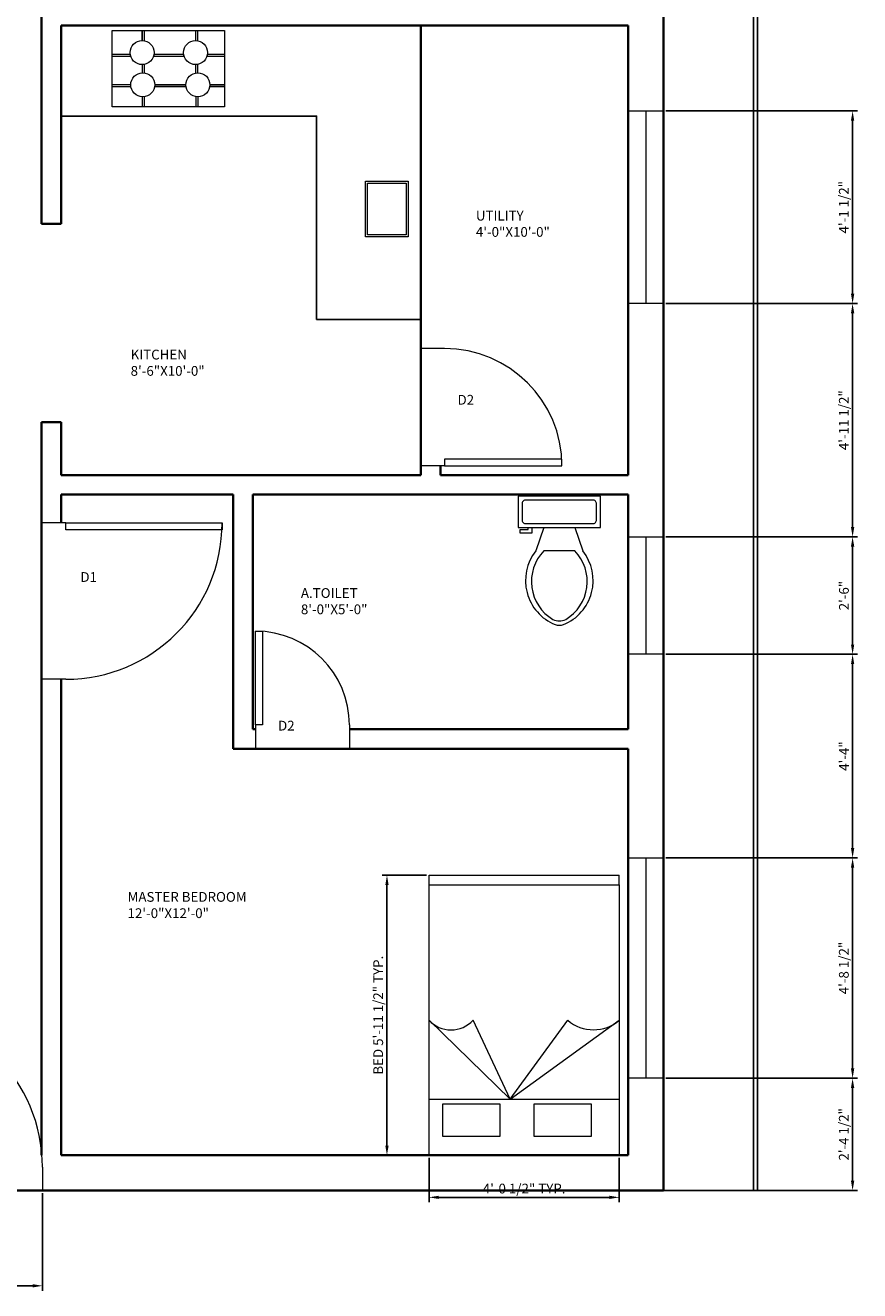
# Model space of a CAD drawing. Units: inches. Extents: x 0 to 3634, y 1847 to 2359.
# Tile 2 of 3: x 3421 to 3634, y 1848 to 2171. Entities that reach past the tile are written whole.
import ezdxf

# ---------------------------------------------------------------- set-up
doc = ezdxf.new("R2010")
doc.units = ezdxf.units.IN
for name, color, linetype, lineweight, true_color in [('A-ANNO-DIMS', 215, 'Continuous', 18, 0xa953a0), ('A-ANNO-TEXT', 215, 'Continuous', 18, 0xa953a0), ('A-AREA-IDEN', 9, 'Continuous', 18, 0xafd9aa), ('A-EQPM', 254, 'Continuous', 18, 0xd7ebd2), ('A-FLOR-CASE', 254, 'Continuous', 25, 0xd7ebd2), ('A-FURN', 254, 'Continuous', 18, 0xd7ebd2), ('A-GLAZ', 9, 'Continuous', 18, 0xafd9aa), ('C-PROP', 9, 'Continuous', 25, 0xafd9aa)]:
    doc.layers.add(name, color=color, linetype=linetype, lineweight=lineweight, true_color=true_color)
for name, color, linetype, lineweight in [('A-DOOR', 4, 'Continuous', 18), ('A-FLOR-FIXT', 9, 'Continuous', 18), ('A-WALL', 7, 'Continuous', 35)]:
    doc.layers.add(name, color=color, linetype=linetype, lineweight=lineweight)
doc.styles.get("Standard").update_dxf_attribs({"font": 'arial.ttf'})
doc.dimstyles.new('ISO-25', dxfattribs={"dimtxt": 2.5, "dimasz": 2.5, "dimexe": 1.25, "dimexo": 0.625, "dimtad": 1, "dimlunit": 3, "dimtxsty": 'Standard', "dimcen": 2.5, "dimadec": 0, "dimazin": 0, "dimtfac": 1, "dimtmove": 0, "dimatfit": 3, "dimfxl": 1, "dimarcsym": 0})

# ---------------------------------------------------------------- blocks, each defined once
blk = doc.blocks.new('*U5')
for p, q in [((9.5, -6), (9.5, -2)), ((-10, -8.5), (-8, -8.5)), ((-10, -9.5), (-10, -8.5)), ((-7, -9.5), (-10, -9.5)), ((-8, -8.5), (-8, -8)), ((-7, -8), (-7, -9.5)), ((-4, -8), (-6, -14)), ((4, -8), (6, -14)), ((4, -14), (-4, -14))]:
    blk.add_line(p, q)
blk.add_lwpolyline([(10.5, -8), (10.5, 0), (-10.5, 0), (-10.5, -8)], close=True)
for points in [[(-9.5, -2), (-9.5, -6)], [(8.5, -1), (-8.5, -1)], [(-8.5, -7), (8.5, -7)]]:
    blk.add_lwpolyline(points)
for centre, radius, start, end in [((-8.62, -1.88), 0.884, 81.8699, 188.1301), ((8.62, -1.88), 0.884, 351.8699, 98.1301), ((-8.62, -6.12), 0.884, 171.8699, 278.1301), ((8.62, -6.12), 0.884, 261.8699, 8.1301), ((3.52, -21.58), 12.17, 141.4691, 247.9714), ((4.2, -21.82), 11.33, 136.3677, 238.9468), ((-3.52, -21.58), 12.17, 292.0284, 38.5307), ((-4.2, -21.82), 11.33, 301.053, 43.6321), ((0, -27.88), 4, 245.7318, 294.2682), ((0, -29), 4, 254.8605, 285.1395)]:
    blk.add_arc(centre, radius, start, end)
blk = doc.blocks.new('*U7')
for p, q in [((0, 0), (0, -6)), ((40, 0), (40, -6))]:
    blk.add_line(p, q)
blk.add_lwpolyline([(0, 0), (0, 40), (1.75, 40), (1.75, 0)], close=True)
blk.add_arc((0, 0), 40, 0, 90)
blk = doc.blocks.new('*U8')
for p, q in [((-30, 0), (-30, -6)), ((0, 0), (0, -6))]:
    blk.add_line(p, q)
blk.add_lwpolyline([(0, 0), (0, 30), (-1.75, 30), (-1.75, 0)], close=True)
blk.add_arc((0, 0), 30, 90, 180)
blk = doc.blocks.new('*U9')
for p, q in [((0, 0), (0, -6)), ((24, 0), (24, -6))]:
    blk.add_line(p, q)
blk.add_lwpolyline([(0, 0), (0, 24), (1.75, 24), (1.75, 0)], close=True)
blk.add_arc((0, 0), 24, 0, 90)
blk = doc.blocks.new('BED-DOUBLE')
for p, q in [((14.39, 48.64), (14.39, 0)), ((34.57, 48.64), (14.39, 27.87)), ((69.14, 48.64), (71.68, 48.64)), ((71.68, 48.64), (71.68, 0)), ((14.39, 27.87), (34.57, 37.39)), ((14.39, 27.87), (34.57, 0)), ((14.39, 27.87), (34.57, 13.18)), ((69.14, 0), (71.68, 0))]:
    blk.add_line(p, q)
for points in [[(0, 48.64), (69.14, 48.64), (69.14, 0), (0, 0)], [(4.78, 45.09), (13.17, 45.09), (13.17, 30.55), (4.78, 30.55)], [(4.78, 21.77), (13.17, 21.77), (13.17, 7.23), (4.78, 7.23)]]:
    blk.add_lwpolyline(points, close=True)
for centre, radius, start, end in [((39.66, 43.02), 7.59, 132.1054, 227.8946), ((42.17, 6.59), 10.06, 139.0804, 220.9196)]:
    blk.add_arc(centre, radius, start, end)
blk = doc.blocks.new('*D20')
at = {"layer": 'A-ANNO-DIMS', "color": 0, "lineweight": -2, "transparency": 16777216}
for p, q in [((3523.45, 1953.98), (3512.07, 1953.98)), ((3513.32, 1884.81), (3513.32, 1951.48)), ((3523.45, 1882.31), (3512.07, 1882.31))]:
    blk.add_line(p, q, dxfattribs=at)
at = {"layer": 'A-ANNO-DIMS', "color": 0, "transparency": 16777216}
for points in [[(3512.9, 1951.48), (3513.74, 1951.48), (3513.32, 1953.98)], [(3512.9, 1884.81), (3513.74, 1884.81), (3513.32, 1882.31)]]:
    blk.add_solid(points, dxfattribs=at)
at = {"layer": 'Defpoints', "color": 0, "transparency": 16777216}
for p in [(3513.32, 1953.98), (3524.07, 1953.98), (3524.07, 1882.31)]:
    blk.add_point(p, dxfattribs=at)
at = {"layer": 'A-ANNO-DIMS', "color": 0, "transparency": 16777216, "insert": (3511.4, 1918.15), "char_height": 2.5, "attachment_point": 5, "rotation": 90}
blk.add_mtext('BED 5\'-11 1/2" TYP.', dxfattribs=at)
blk = doc.blocks.new('*D21')
at = {"layer": 'A-ANNO-DIMS', "color": 0, "lineweight": -2, "transparency": 16777216}
for p, q in [((3524.07, 1881.68), (3524.07, 1870.31)), ((3572.71, 1881.68), (3572.71, 1870.31)), ((3570.21, 1871.56), (3526.57, 1871.56))]:
    blk.add_line(p, q, dxfattribs=at)
at = {"layer": 'A-ANNO-DIMS', "color": 0, "transparency": 16777216}
for points in [[(3526.57, 1871.97), (3526.57, 1871.14), (3524.07, 1871.56)], [(3570.21, 1871.97), (3570.21, 1871.14), (3572.71, 1871.56)]]:
    blk.add_solid(points, dxfattribs=at)
at = {"layer": 'Defpoints', "color": 0, "transparency": 16777216}
for p in [(3524.07, 1882.31), (3572.71, 1882.31), (3524.07, 1871.56)]:
    blk.add_point(p, dxfattribs=at)
at = {"layer": 'A-ANNO-DIMS', "color": 0, "transparency": 16777216, "insert": (3548.39, 1873.48), "char_height": 2.5, "attachment_point": 5}
blk.add_mtext('4\'-0 1/2" TYP.', dxfattribs=at)
blk = doc.blocks.new('*D28')
at = {"layer": 'A-ANNO-DIMS', "color": 0, "lineweight": -2, "transparency": 16777216}
for p, q in [((3385.24, 1872.66), (3385.24, 1847.68)), ((3425.24, 1872.66), (3425.24, 1847.68)), ((3387.74, 1848.93), (3422.74, 1848.93))]:
    blk.add_line(p, q, dxfattribs=at)
at = {"layer": 'A-ANNO-DIMS', "color": 0, "transparency": 16777216}
for points in [[(3387.74, 1849.35), (3387.74, 1848.52), (3385.24, 1848.93)], [(3422.74, 1849.35), (3422.74, 1848.52), (3425.24, 1848.93)]]:
    blk.add_solid(points, dxfattribs=at)
at = {"layer": 'Defpoints', "color": 0, "transparency": 16777216}
for p in [(3385.24, 1873.28), (3425.24, 1873.28), (3425.24, 1848.93)]:
    blk.add_point(p, dxfattribs=at)
at = {"layer": 'A-ANNO-DIMS', "color": 0, "transparency": 16777216, "insert": (3405.24, 1850.84), "char_height": 2.5, "attachment_point": 5}
blk.add_mtext('3\'-4"', dxfattribs=at)
blk = doc.blocks.new('*D38')
at = {"layer": 'A-ANNO-DIMS', "color": 0, "lineweight": -2, "transparency": 16777216}
for p, q in [((3584.64, 2149.44), (3633.62, 2149.44)), ((3632.37, 2102.67), (3632.37, 2146.94)), ((3584.64, 2100.17), (3633.62, 2100.17))]:
    blk.add_line(p, q, dxfattribs=at)
at = {"layer": 'A-ANNO-DIMS', "color": 0, "transparency": 16777216}
for points in [[(3631.95, 2146.94), (3632.79, 2146.94), (3632.37, 2149.44)], [(3631.95, 2102.67), (3632.79, 2102.67), (3632.37, 2100.17)]]:
    blk.add_solid(points, dxfattribs=at)
at = {"layer": 'Defpoints', "color": 0, "transparency": 16777216}
for p in [(3584.02, 2149.44), (3632.37, 2149.44), (3584.02, 2100.17)]:
    blk.add_point(p, dxfattribs=at)
at = {"layer": 'A-ANNO-DIMS', "color": 0, "transparency": 16777216, "insert": (3630.45, 2124.8), "char_height": 2.5, "attachment_point": 5, "rotation": 90}
blk.add_mtext('4\'-1 1/2"', dxfattribs=at)
blk = doc.blocks.new('*D39')
at = {"layer": 'A-ANNO-DIMS', "color": 0, "lineweight": -2, "transparency": 16777216}
for p, q in [((3584.64, 2100.17), (3633.62, 2100.17)), ((3632.37, 2042.99), (3632.37, 2097.67)), ((3584.64, 2040.49), (3633.62, 2040.49))]:
    blk.add_line(p, q, dxfattribs=at)
at = {"layer": 'A-ANNO-DIMS', "color": 0, "transparency": 16777216}
for points in [[(3631.95, 2097.67), (3632.79, 2097.67), (3632.37, 2100.17)], [(3631.95, 2042.99), (3632.79, 2042.99), (3632.37, 2040.49)]]:
    blk.add_solid(points, dxfattribs=at)
at = {"layer": 'Defpoints', "color": 0, "transparency": 16777216}
for p in [(3584.02, 2100.17), (3632.37, 2100.17), (3584.02, 2040.49)]:
    blk.add_point(p, dxfattribs=at)
at = {"layer": 'A-ANNO-DIMS', "color": 0, "transparency": 16777216, "insert": (3630.45, 2070.33), "char_height": 2.5, "attachment_point": 5, "rotation": 90}
blk.add_mtext('4\'-11 1/2"', dxfattribs=at)
blk = doc.blocks.new('*D40')
at = {"layer": 'A-ANNO-DIMS', "color": 0, "lineweight": -2, "transparency": 16777216}
for p, q in [((3584.64, 2040.49), (3633.62, 2040.49)), ((3632.37, 2012.95), (3632.37, 2037.99)), ((3584.64, 2010.45), (3633.62, 2010.45))]:
    blk.add_line(p, q, dxfattribs=at)
at = {"layer": 'A-ANNO-DIMS', "color": 0, "transparency": 16777216}
for points in [[(3631.95, 2037.99), (3632.79, 2037.99), (3632.37, 2040.49)], [(3631.95, 2012.95), (3632.79, 2012.95), (3632.37, 2010.45)]]:
    blk.add_solid(points, dxfattribs=at)
at = {"layer": 'Defpoints', "color": 0, "transparency": 16777216}
for p in [(3584.02, 2040.49), (3632.37, 2040.49), (3584.02, 2010.45)]:
    blk.add_point(p, dxfattribs=at)
at = {"layer": 'A-ANNO-DIMS', "color": 0, "transparency": 16777216, "insert": (3630.47, 2025.47), "char_height": 2.5, "attachment_point": 5, "rotation": 90}
blk.add_mtext('2\'-6"', dxfattribs=at)
blk = doc.blocks.new('*D41')
at = {"layer": 'A-ANNO-DIMS', "color": 0, "lineweight": -2, "transparency": 16777216}
for p, q in [((3584.64, 2010.45), (3633.62, 2010.45)), ((3632.37, 1960.88), (3632.37, 2007.95)), ((3584.64, 1958.38), (3633.62, 1958.38))]:
    blk.add_line(p, q, dxfattribs=at)
at = {"layer": 'A-ANNO-DIMS', "color": 0, "transparency": 16777216}
for points in [[(3631.95, 2007.95), (3632.79, 2007.95), (3632.37, 2010.45)], [(3631.95, 1960.88), (3632.79, 1960.88), (3632.37, 1958.38)]]:
    blk.add_solid(points, dxfattribs=at)
at = {"layer": 'Defpoints', "color": 0, "transparency": 16777216}
for p in [(3584.02, 2010.45), (3632.37, 2010.45), (3584.02, 1958.38)]:
    blk.add_point(p, dxfattribs=at)
at = {"layer": 'A-ANNO-DIMS', "color": 0, "transparency": 16777216, "insert": (3630.49, 1984.42), "char_height": 2.5, "attachment_point": 5, "rotation": 90}
blk.add_mtext('4\'-4"', dxfattribs=at)
blk = doc.blocks.new('*D42')
at = {"layer": 'A-ANNO-DIMS', "color": 0, "lineweight": -2, "transparency": 16777216}
for p, q in [((3584.64, 1958.38), (3633.62, 1958.38)), ((3632.37, 1904.53), (3632.37, 1955.88)), ((3584.64, 1902.03), (3633.62, 1902.03))]:
    blk.add_line(p, q, dxfattribs=at)
at = {"layer": 'A-ANNO-DIMS', "color": 0, "transparency": 16777216}
for points in [[(3631.95, 1955.88), (3632.79, 1955.88), (3632.37, 1958.38)], [(3631.95, 1904.53), (3632.79, 1904.53), (3632.37, 1902.03)]]:
    blk.add_solid(points, dxfattribs=at)
at = {"layer": 'Defpoints', "color": 0, "transparency": 16777216}
for p in [(3584.02, 1958.38), (3632.37, 1958.38), (3584.02, 1902.03)]:
    blk.add_point(p, dxfattribs=at)
at = {"layer": 'A-ANNO-DIMS', "color": 0, "transparency": 16777216, "insert": (3630.45, 1930.21), "char_height": 2.5, "attachment_point": 5, "rotation": 90}
blk.add_mtext('4\'-8 1/2"', dxfattribs=at)
blk = doc.blocks.new('*D43')
at = {"layer": 'A-ANNO-DIMS', "color": 0, "lineweight": -2, "transparency": 16777216}
for p, q in [((3584.64, 1902.03), (3633.62, 1902.03)), ((3632.37, 1875.81), (3632.37, 1899.53)), ((3584.64, 1873.31), (3633.62, 1873.31))]:
    blk.add_line(p, q, dxfattribs=at)
at = {"layer": 'A-ANNO-DIMS', "color": 0, "transparency": 16777216}
for points in [[(3631.95, 1899.53), (3632.79, 1899.53), (3632.37, 1902.03)], [(3631.95, 1875.81), (3632.79, 1875.81), (3632.37, 1873.31)]]:
    blk.add_solid(points, dxfattribs=at)
at = {"layer": 'Defpoints', "color": 0, "transparency": 16777216}
for p in [(3584.02, 1902.03), (3632.37, 1902.03), (3584.02, 1873.31)]:
    blk.add_point(p, dxfattribs=at)
at = {"layer": 'A-ANNO-DIMS', "color": 0, "transparency": 16777216, "insert": (3630.45, 1887.67), "char_height": 2.5, "attachment_point": 5, "rotation": 90}
blk.add_mtext('2\'-4 1/2"', dxfattribs=at)

msp = doc.modelspace()

# ---------------------------------------------------------------- linework, layer by layer
at = {"layer": 'A-EQPM'}
for p, q in [((3450.715, 2167.425), (3450.715, 2169.965)), ((3450.715, 2169.965), (3450.715, 2167.425)), ((3451.215, 2169.965), (3451.215, 2167.384)), ((3464.47, 2167.424), (3464.47, 2169.965)), ((3464.97, 2167.367), (3464.97, 2169.965)), ((3443.062, 2163.923), (3447.675, 2163.923)), ((3443.062, 2163.423), (3447.789, 2163.423)), ((3453.641, 2163.423), (3461.451, 2163.423)), ((3453.755, 2163.923), (3461.337, 2163.923)), ((3467.303, 2163.423), (3471.768, 2163.423)), ((3467.417, 2163.923), (3471.768, 2163.923)), ((3450.715, 2161.283), (3450.715, 2159.19)), ((3451.215, 2161.324), (3451.215, 2159.177)), ((3464.47, 2159.154), (3464.47, 2161.285)), ((3464.97, 2159.195), (3464.97, 2161.341)), ((3447.809, 2156.124), (3443.062, 2156.124)), ((3447.85, 2155.624), (3443.062, 2155.624)), ((3461.94, 2155.624), (3453.91, 2155.624)), ((3461.899, 2156.124), (3453.951, 2156.124)), ((3453.951, 2156.124), (3461.899, 2156.124)), ((3471.768, 2155.624), (3468, 2155.624)), ((3471.768, 2156.124), (3468.041, 2156.124)), ((3468.041, 2156.124), (3471.768, 2156.124)), ((3450.715, 2153.058), (3450.715, 2150.474)), ((3451.215, 2153.072), (3451.215, 2150.474)), ((3464.47, 2153.053), (3464.47, 2153.094)), ((3464.47, 2153.094), (3464.47, 2150.474)), ((3464.97, 2153.053), (3464.97, 2150.474))]:
    msp.add_line(p, q, dxfattribs=at)
msp.add_lwpolyline([(3443.062, 2169.965), (3471.768, 2169.965), (3471.768, 2150.474), (3443.062, 2150.474)], close=True, dxfattribs=at)
for centre in [(3450.715, 2164.354), (3464.377, 2164.354), (3450.88, 2156.124), (3464.97, 2156.124)]:
    msp.add_circle(centre, 3.071, dxfattribs=at)
at = {"layer": 'A-FLOR-CASE'}
msp.add_lwpolyline([(3430.018, 2148.132), (3495.324, 2148.132), (3495.324, 2096.095), (3522.018, 2096.095)], dxfattribs=at)
at = {"layer": 'A-FLOR-FIXT'}
for points in [[(3507.827, 2131.461), (3518.71, 2131.461), (3518.71, 2117.219), (3507.827, 2117.219)], [(3508.327, 2130.961), (3518.21, 2130.961), (3518.21, 2117.719), (3508.327, 2117.719)]]:
    msp.add_lwpolyline(points, close=True, dxfattribs=at)
at = {"layer": 'A-GLAZ'}
for p, q in [((3575.018, 2149.437), (3584.018, 2149.437)), ((3575.018, 2100.167), (3575.018, 2149.437)), ((3575.018, 2149.437), (3579.518, 2149.437)), ((3579.518, 2149.437), (3579.518, 2100.167)), ((3584.018, 2149.437), (3584.018, 2100.167)), ((3584.018, 2100.167), (3575.018, 2100.167)), ((3575.018, 2040.491), (3584.018, 2040.491)), ((3575.018, 2010.448), (3575.018, 2040.491)), ((3575.018, 2040.491), (3579.518, 2040.491)), ((3579.518, 2040.491), (3579.518, 2010.448)), ((3584.018, 2040.491), (3584.018, 2010.448)), ((3584.018, 2010.448), (3575.018, 2010.448)), ((3575.018, 1958.383), (3584.018, 1958.383)), ((3575.018, 1902.029), (3575.018, 1958.383)), ((3575.018, 1958.383), (3579.518, 1958.383)), ((3579.518, 1958.383), (3579.518, 1902.029)), ((3584.018, 1958.383), (3584.018, 1902.029)), ((3584.018, 1902.029), (3575.018, 1902.029))]:
    msp.add_line(p, q, dxfattribs=at)
at = {"layer": 'A-WALL'}
for p, q in [((3584.018, 2305.309), (3584.018, 1873.309)), ((3425.018, 2176.309), (3425.018, 2120.548)), ((3430.018, 2171.309), (3522.018, 2171.309)), ((3430.018, 2171.309), (3430.018, 2120.548)), ((3522.018, 2171.309), (3522.018, 2056.309)), ((3522.018, 2171.309), (3575.018, 2171.309)), ((3575.018, 2171.309), (3575.018, 2056.309)), ((3425.018, 2120.548), (3430.018, 2120.548)), ((3425.018, 2069.854), (3430.018, 2069.854)), ((3425.018, 2069.854), (3425.018, 1882.309)), ((3430.018, 2069.854), (3430.018, 2056.309)), ((3527.018, 2058.654), (3527.018, 2056.309)), ((3430.018, 2056.309), (3522.018, 2056.309)), ((3527.018, 2056.309), (3575.018, 2056.309)), ((3430.018, 2051.309), (3474.018, 2051.309)), ((3430.018, 2051.309), (3430.018, 2044.056)), ((3461.018, 2051.309), (3466.018, 2051.309)), ((3474.018, 2051.309), (3474.018, 1986.309)), ((3479.018, 2051.309), (3479.018, 1991.309)), ((3479.018, 2051.309), (3575.018, 2051.309)), ((3575.018, 2051.309), (3575.018, 1991.309)), ((3430.018, 2004.056), (3430.018, 1882.309)), ((3479.018, 1991.309), (3479.713, 1991.309)), ((3503.713, 1991.309), (3575.018, 1991.309)), ((3474.018, 1986.309), (3575.018, 1986.309)), ((3575.018, 1986.309), (3575.018, 1882.309)), ((3575.018, 1882.309), (3430.018, 1882.309)), ((3584.018, 1873.309), (3272.018, 1873.309))]:
    msp.add_line(p, q, dxfattribs=at)
at = {"layer": 'C-PROP'}
for p, q in [((3607.018, 2305.309), (3607.018, 1873.309)), ((3608.018, 2305.309), (3608.018, 1873.309)), ((3608.018, 1873.309), (3584.018, 1873.309))]:
    msp.add_line(p, q, dxfattribs=at)

# ---------------------------------------------------------------- block references
at = {"layer": 'A-DOOR', "rotation": 270}
for name, p in [('*U8', (3528.07, 2058.654)), ('*U7', (3431.177, 2044.056))]:
    msp.add_blockref(name, p, dxfattribs=at)
at = {"layer": 'A-DOOR'}
for name, p in [('*U9', (3479.713, 1992.379)), ('*U7', (3385.237, 1879.283))]:
    msp.add_blockref(name, p, dxfattribs=at)
at = {"layer": 'A-FLOR-FIXT'}
msp.add_blockref('*U5', (3557.384, 2050.896), dxfattribs=at)
at = {"layer": 'A-FURN', "rotation": 90.0000000000009}
msp.add_blockref('BED-DOUBLE', (3572.715, 1882.309), dxfattribs=at)

# ---------------------------------------------------------------- texts
at = {"layer": 'A-ANNO-TEXT', "char_height": 2.5, "attachment_point": 1}
for s, width, insert in [('D2', 14.79582, (3531.36, 2076.797)), ('D1', 11.25576, (3434.934, 2031.471)), ('D2', 7.94872, (3485.472, 1993.457))]:
    msp.add_mtext_dynamic_manual_height_columns(s, width=width, gutter_width=12.5, heights=[0], dxfattribs=dict(at, insert=insert))
at = {"layer": 'A-AREA-IDEN', "char_height": 2.5, "attachment_point": 1}
for s, width, insert in [('UTILITY\\P4\'-0"X10\'-0"', 28.5841, (3536.053, 2123.904)), ('KITCHEN\\P8\'-6"X10\'-0"', 53.28483, (3447.787, 2088.359)), ('A.TOILET\\P8\'-0"X5\'-0"', 40.84234, (3491.312, 2027.375)), ('MASTER BEDROOM\\P12\'-0"X12\'-0"', 60.74089, (3446.995, 1949.658))]:
    msp.add_mtext_dynamic_manual_height_columns(s, width=width, gutter_width=12.5, heights=[0], dxfattribs=dict(at, insert=insert))

# ---------------------------------------------------------------- dimensions: what is measured, and where the dimension line sits
at = {"layer": 'A-ANNO-DIMS'}
for base, p1, p2, picture, middle in [((3632.368, 2149.437), (3584.018, 2100.167), (3584.018, 2149.437), '*D38', (3630.451, 2124.802)), ((3632.368, 2100.167), (3584.018, 2040.491), (3584.018, 2100.167), '*D39', (3630.451, 2070.329)), ((3632.368, 2040.491), (3584.018, 2010.448), (3584.018, 2040.491), '*D40', (3630.467, 2025.47)), ((3632.368, 2010.448), (3584.018, 1958.383), (3584.018, 2010.448), '*D41', (3630.493, 1984.416)), ((3632.368, 1958.383), (3584.018, 1902.029), (3584.018, 1958.383), '*D42', (3630.451, 1930.206)), ((3632.368, 1902.029), (3584.018, 1873.309), (3584.018, 1902.029), '*D43', (3630.451, 1887.669))]:
    dim = msp.add_linear_dim(base=base, p1=p1, p2=p2, angle=90, dimstyle='ISO-25', override={"dimdec": 1, "dimlfac": 1, "dimrnd": 0, "dimzin": 1, "dimdsep": 46, "dimlunit": 4, "dimfrac": 2}, dxfattribs=at)
    dim.commit()
    dim.dimension.update_dxf_attribs({"geometry": picture, "text_midpoint": middle})
for base, p1, p2, angle, text, picture, middle in [((3513.319, 1953.985), (3524.071, 1882.309), (3524.071, 1953.985), 90, 'BED <> TYP.', '*D20', (3511.402, 1918.147)), ((3524.071, 1871.558), (3572.715, 1882.309), (3524.071, 1882.309), 180, '<> TYP.', '*D21', (3548.393, 1873.475))]:
    dim = msp.add_linear_dim(base=base, p1=p1, p2=p2, angle=angle, text=text, dimstyle='ISO-25', override={"dimdec": 1, "dimlfac": 1, "dimrnd": 0, "dimzin": 1, "dimdsep": 46, "dimlunit": 4, "dimfrac": 2}, dxfattribs=at)
    dim.commit()
    dim.dimension.update_dxf_attribs({"geometry": picture, "text_midpoint": middle})
dim = msp.add_linear_dim(base=(3425.237, 1848.933), p1=(3385.237, 1873.283), p2=(3425.237, 1873.283), dimstyle='ISO-25', override={"dimdec": 1, "dimlfac": 1, "dimrnd": 0, "dimzin": 1, "dimdsep": 46, "dimlunit": 4, "dimfrac": 2}, dxfattribs=at)
dim.commit()
dim.dimension.update_dxf_attribs({"geometry": '*D28', "text_midpoint": (3405.237, 1850.836)})

doc.saveas('drawing.dxf')
